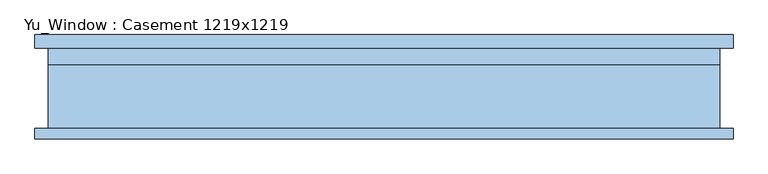
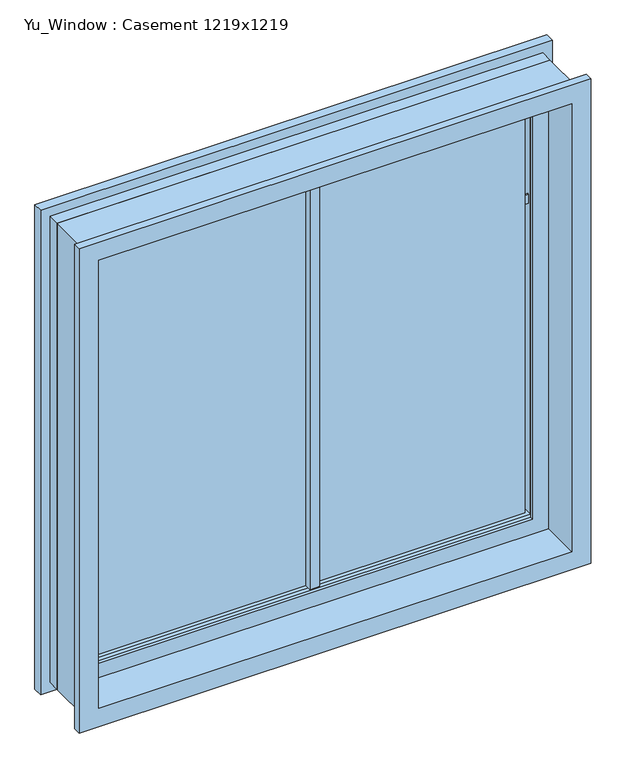
"""IFC4 building model written with IfcOpenShell, lengths in millimetres: window geometry, Yu_Window : Casement 1219x1219."""

from ifc_helpers import new_model, si_unit, frame, origin, place, context, project, spatial, polyline, outline, extrude, faceted_brep, source, transform, mapped, element, save


def yu_window_casement_1219x1219_b0d26e5b(model_context):
    return source(origin(), model_context, "Body", "SolidModel", [
        faceted_brep([(584.6, 23.8, 1794.2), (584.6, 43.8, 1794.2), (584.6, 43.8, 625.0), (584.6, 23.8, 625.0), (634.6, 43.8, 1844.2), (634.6, 43.8, 575.0), (-634.6, 43.8, 575.0), (-634.6, 43.8, 1844.2), (-584.6, 43.8, 1794.2), (-584.6, 43.8, 625.0), (-584.6, 23.8, 625.0), (-609.6, 23.8, 1819.2), (-609.6, 23.8, 600.0), (609.6, 23.8, 600.0), (609.6, 23.8, 1819.2), (-584.6, 23.8, 1794.2), (609.6, -96.2, 1819.2), (609.6, -96.2, 600.0), (-609.6, -96.2, 600.0), (-659.6, -96.2, 1869.2), (-659.6, -96.2, 550.0), (659.6, -96.2, 550.0), (659.6, -96.2, 1869.2), (-609.6, -96.2, 1819.2), (659.6, -76.2, 1869.2), (659.6, -76.2, 550.0), (-659.6, -76.2, 550.0), (-659.6, -76.2, 1869.2), (-634.6, -76.2, 1844.2), (-634.6, -76.2, 575.0), (634.6, -76.2, 575.0), (634.6, -76.2, 1844.2)], [[[0, 1, 2, 3]], [[4, 5, 6, 7], [8, 9, 2, 1]], [[3, 2, 9, 10]], [[11, 12, 13, 14], [0, 3, 10, 15]], [[16, 14, 13, 17]], [[17, 13, 12, 18]], [[19, 20, 21, 22], [16, 17, 18, 23]], [[24, 22, 21, 25]], [[25, 21, 20, 26]], [[24, 25, 26, 27], [28, 29, 30, 31]], [[4, 31, 30, 5]], [[5, 30, 29, 6]], [[10, 9, 8, 15]], [[18, 12, 11, 23]], [[26, 20, 19, 27]], [[6, 29, 28, 7]], [[15, 8, 1, 0]], [[23, 11, 14, 16]], [[27, 19, 22, 24]], [[7, 28, 31, 4]]]),
        faceted_brep([(-584.6, 68.8, 1794.2), (-584.6, 43.8, 1794.2), (-584.6, 43.8, 625.0), (-584.6, 68.8, 625.0), (-634.6, 43.8, 1844.2), (-634.6, 43.8, 575.0), (634.6, 43.8, 575.0), (634.6, 43.8, 1844.2), (584.6, 43.8, 1794.2), (584.6, 43.8, 625.0), (584.6, 68.8, 625.0), (609.6, 68.8, 1819.2), (609.6, 68.8, 600.0), (-609.6, 68.8, 600.0), (-609.6, 68.8, 1819.2), (584.6, 68.8, 1794.2), (-609.6, 101.2, 1819.2), (-609.6, 101.2, 600.0), (609.6, 101.2, 600.0), (659.6, 101.2, 1869.2), (659.6, 101.2, 550.0), (-659.6, 101.2, 550.0), (-659.6, 101.2, 1869.2), (609.6, 101.2, 1819.2), (-659.6, 76.2, 1869.2), (-659.6, 76.2, 550.0), (659.6, 76.2, 550.0), (659.6, 76.2, 1869.2), (634.6, 76.2, 1844.2), (634.6, 76.2, 575.0), (-634.6, 76.2, 575.0), (-634.6, 76.2, 1844.2)], [[[0, 1, 2, 3]], [[4, 5, 6, 7], [8, 9, 2, 1]], [[3, 2, 9, 10]], [[11, 12, 13, 14], [0, 3, 10, 15]], [[16, 14, 13, 17]], [[17, 13, 12, 18]], [[19, 20, 21, 22], [16, 17, 18, 23]], [[24, 22, 21, 25]], [[25, 21, 20, 26]], [[24, 25, 26, 27], [28, 29, 30, 31]], [[4, 31, 30, 5]], [[5, 30, 29, 6]], [[10, 9, 8, 15]], [[18, 12, 11, 23]], [[26, 20, 19, 27]], [[6, 29, 28, 7]], [[15, 8, 1, 0]], [[23, 11, 14, 16]], [[27, 19, 22, 24]], [[7, 28, 31, 4]]]),
        extrude(outline(polyline([(605.0, 604.6), (1814.2, 604.6), (1814.2, -604.6), (605.0, -604.6), (605.0, 604.6)]), holes=[polyline([(645.0, -564.6), (1774.2, -564.6), (1774.2, 564.6), (645.0, 564.6), (645.0, -564.6)])]), frame((0.0, 0.0, 0.0), z_axis=(0.0, 1.0, 0.0), x_axis=(0.0, 0.0, 1.0)), (0.0, 0.0, 1.0), 8.8),
        extrude(outline(polyline([(605.0, 604.6), (1814.2, 604.6), (1814.2, -604.6), (605.0, -604.6), (605.0, 604.6)]), holes=[polyline([(655.0, -554.6), (1764.2, -554.6), (1764.2, 554.6), (655.0, 554.6), (655.0, -554.6)])]), frame((0.0, 68.8, 0.0), z_axis=(0.0, 1.0, 0.0), x_axis=(0.0, 0.0, 1.0)), (0.0, 0.0, 1.0), 15.0),
        extrude(outline(polyline([(-554.6, 22.0), (554.6, 22.0), (554.6, 18.0), (-554.6, 18.0), (-554.6, 22.0)])), frame((0.0, 0.0, 655.0), z_axis=(0.0, 0.0, 1.0), x_axis=(1.0, 0.0, 0.0)), (0.0, 0.0, 1.0), 1109.2),
        extrude(outline(polyline([(15.4, 68.8), (15.4, 0.0), (-9.6, 0.0), (-9.6, 68.8), (15.4, 68.8)])), frame((0.0, 0.0, 655.0), z_axis=(0.0, 0.0, 1.0), x_axis=(1.0, 0.0, 0.0)), (0.0, 0.0, 1.0), 1159.2),
        extrude(outline(polyline([(-564.6, 18.0), (-564.6, 22.0), (564.6, 22.0), (564.6, 18.0), (-564.6, 18.0)])), frame((0.0, 0.0, 1494.2), z_axis=(0.0, 0.0, 1.0), x_axis=(1.0, 0.0, 0.0)), (0.0, 0.0, 1.0), 25.0),
    ])


if __name__ == "__main__":
    model = new_model("IFC4")
    model_context = context("Model", 3, world=origin())
    ifc_project = project(units=[si_unit("LENGTHUNIT", "METRE", prefix="MILLI")], contexts=[model_context])
    site = spatial("IfcSite", under=ifc_project)
    building = spatial("IfcBuilding", under=site)
    placement = place(None, origin())
    yu_window_casement_1219x1219_shape = yu_window_casement_1219x1219_b0d26e5b(model_context)
    element("IfcWindow", 1, ObjectType="Yu_Window : Casement 1219x1219", at=placement, inside=building, context=model_context, shape_type="MappedRepresentation", body=[
        mapped(yu_window_casement_1219x1219_shape, transform((0.0, 0.0, 0.0), x_axis=(1.0, 0.0, 0.0), y_axis=(0.0, 1.0, 0.0), z_axis=(0.0, 0.0, 1.0))),
    ])
    save(model, "model.ifc")

# Revit data of these elements
# Type "Yu_Window : Casement 1219x1219"
#   Type Mark = "22"
#   Analytic Construction = "<None>"
#   mullion 2 = 0' - 11.81102"
#   Window panel size 1 = 1' - 11.62205"
#   Offset = 0' - 0.98425"
#   Height = 4' - 0"
#   Default Sill Height = 1' - 11.62205"
#   Width = 4' - 0"
#   Define Thermal Properties by = 1
#   Interior material = none
#   Exterior material = none
#   Wall Closure = (empty or 0)
# Element 1 (IfcWindow, "Yu_Window : Casement 1219x1219")
#   Materials on its faces: "Glass"
# Materials
#   "Glass": class "Glass", colour RGB 0 128 192, transparency 0.75, Description = "Soda Lime Glass", Cost = 0
